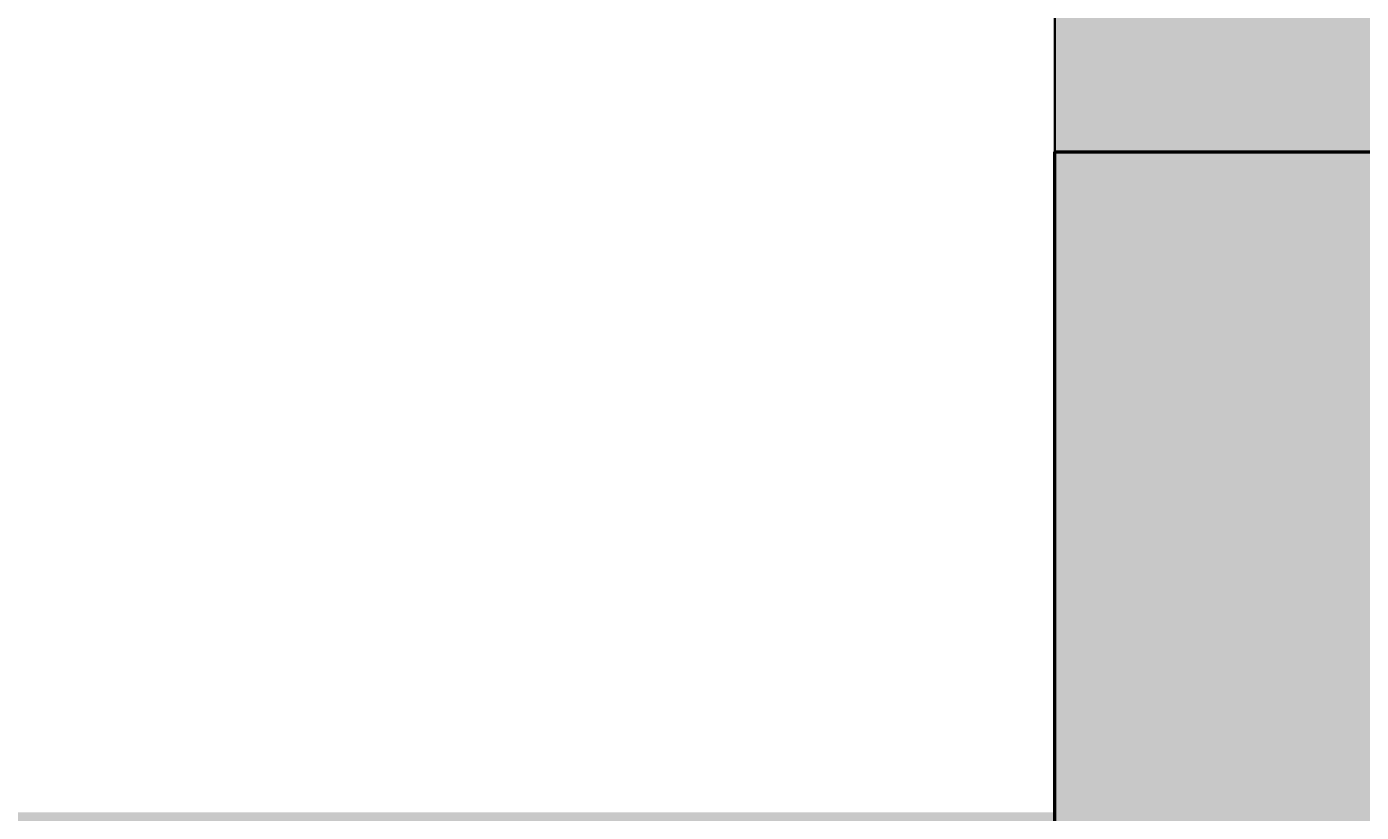
# Model space of a CAD drawing. Units: inches. Extents: x 1998 to 2588, y 1139 to 1977.
# Tile 60 of 134: x 2063 to 2095, y 1760 to 1779. Entities that reach past the tile are written whole.
import ezdxf

# ---------------------------------------------------------------- set-up
doc = ezdxf.new("R2010")
doc.units = ezdxf.units.IN
for name, color, linetype, lineweight in [('A-ANNO-DIMS', 2, 'Continuous', 18), ('A-COLS-PATT', 250, 'Continuous', 13), ('A-WALL-PATT', 252, 'Continuous', 13), ('COLUMN', 10, 'Continuous', 50), ('WALL', 200, 'Continuous', 35)]:
    doc.layers.add(name, color=color, linetype=linetype, lineweight=lineweight)
doc.styles.get("Standard").update_dxf_attribs({"font": 'arial.ttf'})
doc.dimstyles.get("Standard").update_dxf_attribs({"dimtxt": 0.18, "dimasz": 0.18, "dimexe": 0.18, "dimexo": 0.0625, "dimgap": 0.09, "dimtad": 0, "dimtih": 1, "dimtoh": 1, "dimdec": 4, "dimzin": 0, "dimdsep": 46, "dimtxsty": 'Standard', "dimcen": 0.09, "dimadec": 0, "dimazin": 0, "dimtfac": 1, "dimtdec": 4, "dimtofl": 0, "dimtmove": 0, "dimatfit": 3, "dimfxl": 1, "dimtolj": 1, "dimtzin": 0, "dimarcsym": 0})

# ---------------------------------------------------------------- blocks, each defined once
blk = doc.blocks.new('*D28')
at = {"layer": 'A-ANNO-DIMS', "color": 0, "lineweight": -2, "transparency": 16777216}
for p, q in [((2059.473, 1759.795), (2059.473, 1977.362)), ((2087.973, 1759.795), (2087.973, 1977.362)), ((2059.653, 1977.182), (2073.397, 1977.182)), ((2087.793, 1977.182), (2074.049, 1977.182))]:
    blk.add_line(p, q, dxfattribs=at)
at = {"layer": 'A-ANNO-DIMS', "color": 0, "transparency": 16777216}
for points in [[(2059.653, 1977.212), (2059.653, 1977.152), (2059.473, 1977.182)], [(2087.793, 1977.212), (2087.793, 1977.152), (2087.973, 1977.182)]]:
    blk.add_solid(points, dxfattribs=at)
at = {"layer": 'Defpoints', "color": 0, "transparency": 16777216}
for p in [(2087.973, 1977.182), (2059.473, 1759.732), (2087.973, 1759.732)]:
    blk.add_point(p, dxfattribs=at)
at = {"layer": 'A-ANNO-DIMS', "color": 0, "transparency": 16777216, "insert": (2073.723, 1977.182), "char_height": 0.18, "attachment_point": 5}
blk.add_mtext('\\A1;28.5', dxfattribs=at)
blk = doc.blocks.new('*D29')
at = {"layer": 'A-ANNO-DIMS', "color": 0, "lineweight": -2, "transparency": 16777216}
for p, q in [((2087.91, 1888.732), (1997.843, 1888.732)), ((1998.023, 1888.552), (1998.023, 1824.414)), ((1998.023, 1759.912), (1998.023, 1824.05)), ((2059.41, 1759.732), (1997.843, 1759.732))]:
    blk.add_line(p, q, dxfattribs=at)
at = {"layer": 'A-ANNO-DIMS', "color": 0, "transparency": 16777216}
for points in [[(1997.993, 1888.552), (1998.053, 1888.552), (1998.023, 1888.732)], [(1997.993, 1759.912), (1998.053, 1759.912), (1998.023, 1759.732)]]:
    blk.add_solid(points, dxfattribs=at)
at = {"layer": 'Defpoints', "color": 0, "transparency": 16777216}
for p in [(1998.023, 1888.732), (2087.973, 1888.732), (2059.473, 1759.732)]:
    blk.add_point(p, dxfattribs=at)
at = {"layer": 'A-ANNO-DIMS', "color": 0, "transparency": 16777216, "insert": (1998.023, 1824.232), "char_height": 0.18, "attachment_point": 5}
blk.add_mtext('\\A1;129', dxfattribs=at)

msp = doc.modelspace()

# ---------------------------------------------------------------- hatches: boundary and pattern name
at = {"layer": 'A-COLS-PATT'}
h = msp.add_hatch(color=256, dxfattribs=at)
h.dxf.hatch_style = 1
h.paths.add_polyline_path([(2099.4125, 1888.7324), (2087.9729, 1888.7324), (2087.9729, 1868.3278), (2099.4125, 1868.3278)])
h.paths.add_polyline_path([(2234.4125, 1888.7324), (2222.9729, 1888.7324), (2222.9729, 1868.3278), (2234.4125, 1868.3278)])
h.paths.add_polyline_path([(2341.4729, 1886.637), (2330.0332, 1886.637), (2330.0332, 1866.2324), (2341.4729, 1866.2324)])
h.paths.add_polyline_path([(2507.8006, 1882.7324), (2487.396, 1882.7324), (2487.396, 1871.2927), (2507.8006, 1871.2927)])
h.paths.add_polyline_path([(2510.9729, 1766.672), (2490.5682, 1766.672), (2490.5682, 1755.2324), (2510.9729, 1755.2324)])
h.paths.add_polyline_path([(2345.9729, 1759.7324), (2334.5332, 1759.7324), (2334.5332, 1739.3278), (2345.9729, 1739.3278)])
h.paths.add_polyline_path([(2234.4125, 1774.3318), (2222.9729, 1774.3318), (2222.9729, 1753.9272), (2234.4125, 1753.9272)])
h.paths.add_polyline_path([(2099.4125, 1775.637), (2087.9729, 1775.637), (2087.9729, 1755.2324), (2099.4125, 1755.2324)])
h.paths.add_polyline_path([(2098.0956, 1593.7241), (2077.691, 1593.7241), (2077.691, 1582.2845), (2098.0956, 1582.2845)])
h.paths.add_polyline_path([(2227.4729, 1604.637), (2216.0332, 1604.637), (2216.0332, 1584.2324), (2227.4729, 1584.2324)])
h.paths.add_polyline_path([(2345.9729, 1647.5211), (2334.5332, 1647.5211), (2334.5332, 1627.1165), (2345.9729, 1627.1165)])
h.paths.add_polyline_path([(2522.3775, 1641.2324), (2501.9729, 1641.2324), (2501.9729, 1629.7927), (2522.3775, 1629.7927)])
h.paths.add_polyline_path([(2522.3775, 1480.7324), (2501.9729, 1480.7324), (2501.9729, 1469.2927), (2522.3775, 1469.2927)])
h.paths.add_polyline_path([(2345.9729, 1488.5616), (2334.5332, 1488.5616), (2334.5332, 1468.1569), (2345.9729, 1468.1569)])
h.paths.add_polyline_path([(2234.4125, 1486.137), (2227.4729, 1486.137), (2227.4729, 1465.7324), (2234.4125, 1465.7324)])
h.paths.add_polyline_path([(2227.4729, 1486.137), (2222.9729, 1486.137), (2222.9729, 1465.7324), (2227.4729, 1465.7324)])
h.paths.add_polyline_path([(2108.3775, 1470.2324), (2087.9729, 1470.2324), (2087.9729, 1458.7927), (2108.3775, 1458.7927)])
h.paths.add_polyline_path([(2096.9729, 1365.5012), (2087.9729, 1365.5012), (2087.9729, 1345.0966), (2096.9729, 1345.0966)])
h.paths.add_polyline_path([(2087.9729, 1365.5012), (2085.5332, 1365.5012), (2085.5332, 1345.0966), (2087.9729, 1345.0966)])
h.paths.add_polyline_path([(2234.4125, 1285.137), (2222.9729, 1285.137), (2222.9729, 1264.7324), (2234.4125, 1264.7324)])
h.paths.add_polyline_path([(2345.9729, 1285.137), (2334.5332, 1285.137), (2334.5332, 1264.7324), (2345.9729, 1264.7324)])
h.paths.add_polyline_path([(2503.1458, 1240.172), (2482.7412, 1240.172), (2482.7412, 1228.7324), (2503.1458, 1228.7324)])
h.paths.add_polyline_path([(2510.9729, 1369.172), (2490.5682, 1369.172), (2490.5682, 1357.7324), (2510.9729, 1357.7324)])
at = {"layer": 'A-WALL-PATT'}
h = msp.add_hatch(color=256, dxfattribs=at)
h.dxf.hatch_style = 1
h.paths.add_polyline_path([(2222.9729, 1888.7324), (2099.4125, 1888.7324), (2099.4125, 1879.7324), (2222.9729, 1879.7324)])
h.paths.add_polyline_path([(2096.9729, 1868.3278), (2087.9729, 1868.3278), (2087.9729, 1775.637), (2096.9729, 1775.637)])
h.paths.add_polyline_path([(2227.4729, 1868.3278), (2222.9729, 1868.3278), (2222.9729, 1774.3318), (2227.4729, 1774.3318)])
h.paths.add_polyline_path([(2188.3019, 1759.7324), (2138.6074, 1759.7324), (2099.4125, 1759.7324), (2099.4125, 1755.2324), (2176.9729, 1755.2324), (2188.3019, 1755.2324)])
h.paths.add_polyline_path([(2087.9729, 1759.7324), (2059.4729, 1759.7324), (2059.4729, 1702.7324), (2087.9729, 1702.7324), (2087.9729, 1707.2324), (2063.9729, 1707.2324), (2063.9729, 1755.2324), (2087.9729, 1755.2324)])
h.paths.add_polyline_path([(2096.9729, 1755.2324), (2087.9729, 1755.2324), (2087.9729, 1707.2324), (2096.9729, 1707.2324)])
h.paths.add_polyline_path([(2187.0461, 1707.2324), (2105.9729, 1707.2324), (2096.9729, 1707.2324), (2087.9729, 1707.2324), (2087.9729, 1702.7324), (2105.9729, 1702.7324), (2114.9729, 1702.7324), (2187.0461, 1702.7324)])
h.paths.add_polyline_path([(2181.4729, 1719.2028), (2176.9729, 1719.2028), (2176.9729, 1707.2324), (2181.4729, 1707.2324)])
h.paths.add_polyline_path([(2216.0332, 1588.7324), (2114.9729, 1588.7324), (2105.9729, 1588.7324), (2105.9729, 1584.2324), (2216.0332, 1584.2324)])
h.paths.add_polyline_path([(2077.691, 1588.7324), (2061.4729, 1588.7324), (2061.4729, 1584.2324), (2077.691, 1584.2324)])
h.paths.add_polyline_path([(2105.9729, 1588.7324), (2098.0956, 1588.7324), (2098.0956, 1584.2324), (2105.9729, 1584.2324)])
h.paths.add_polyline_path([(2114.9729, 1596.2642), (2110.1012, 1596.2642), (2105.9729, 1596.2642), (2105.9729, 1588.7324), (2114.9729, 1588.7324)])
h.paths.add_polyline_path([(2114.9729, 1584.2324), (2105.9729, 1584.2324), (2105.9729, 1580.249), (2110.1012, 1580.249), (2114.9729, 1580.249)])
h.paths.add_polyline_path([(2114.9729, 1547.7716), (2110.1012, 1547.7716, -0.0318759), (2105.9729, 1548.035), (2105.9729, 1470.2324), (2108.3775, 1470.2324), (2108.3775, 1465.7324), (2186.2943, 1465.7324), (2186.2943, 1470.2324), (2114.9729, 1470.2324)])
h.paths.add_polyline_path([(2227.4729, 1584.2324), (2222.9729, 1584.2324), (2222.9729, 1486.137), (2227.4729, 1486.137)])
h.paths.add_polyline_path([(2295.4138, 1593.2324), (2227.4729, 1593.2324), (2227.4729, 1588.7324), (2295.4138, 1588.7324), (2295.4138, 1591.8729)])
h.paths.add_polyline_path([(2345.9729, 1627.1165), (2341.4729, 1627.1165), (2341.4729, 1593.2324), (2337.2869, 1593.2324), (2337.2869, 1591.8729), (2337.2869, 1588.7324), (2345.9729, 1588.7324)])
h.paths.add_polyline_path([(2291.9729, 1588.7324), (2287.4729, 1588.7324), (2287.4729, 1522.7324), (2291.9729, 1522.7324)])
h.paths.add_polyline_path([(2291.9729, 1522.7324), (2287.4729, 1522.7324), (2227.4729, 1522.7324), (2227.4729, 1518.2324), (2291.9729, 1518.2324)])
h.paths.add_polyline_path([(2295.7347, 1519.5919), (2295.7347, 1522.7324), (2291.9729, 1522.7324), (2291.9729, 1518.2324), (2295.7347, 1518.2324)])
h.paths.add_polyline_path([(2345.9729, 1522.7324), (2337.6078, 1522.7324), (2337.6078, 1519.5919), (2337.6078, 1518.2324), (2341.4729, 1518.2324), (2341.4729, 1488.5616), (2345.9729, 1488.5616)])
h.paths.add_polyline_path([(2345.9729, 1468.1569), (2341.4729, 1468.1569), (2341.4729, 1374.2324), (2227.4729, 1374.2324), (2227.4729, 1369.7324), (2345.9729, 1369.7324)])
h.paths.add_polyline_path([(2345.9729, 1369.7324), (2341.4729, 1369.7324), (2341.4729, 1362.2324), (2345.9729, 1362.2324)])
h.paths.add_polyline_path([(2345.9729, 1317.7324), (2345.9729, 1322.2324), (2341.4729, 1322.2324), (2341.4729, 1285.137), (2345.9729, 1285.137)], flags=17)
h.paths.add_polyline_path([(2356.2096, 1322.2324), (2345.9729, 1322.2324), (2345.9729, 1317.7324), (2356.2096, 1317.7324), (2356.2096, 1319.3088)], flags=17)
h.paths.add_polyline_path([(2393.9729, 1322.2324), (2375.6999, 1322.2324), (2375.6999, 1319.3088, -0.0202458), (2375.636, 1317.7324), (2393.9729, 1317.7324)], flags=17)
h.paths.add_polyline_path([(2398.4729, 1322.2324), (2393.9729, 1322.2324), (2393.9729, 1317.7324), (2393.9729, 1237.7324), (2345.9729, 1237.7324), (2345.9729, 1264.7324), (2341.4729, 1264.7324), (2341.4729, 1228.7324), (2393.9729, 1228.7324), (2482.7412, 1228.7324), (2482.7412, 1237.7324), (2398.4729, 1237.7324), (2398.4729, 1297.1029)])
h.paths.add_polyline_path([(2398.4729, 1362.2324), (2393.9729, 1362.2324), (2393.9729, 1357.7324), (2398.4729, 1357.7324)])
h.paths.add_polyline_path([(2345.9729, 1329.7549), (2341.4729, 1329.7549), (2341.4729, 1322.2324), (2345.9729, 1322.2324)])

# ---------------------------------------------------------------- linework, layer by layer
at = {"layer": 'COLUMN'}
msp.add_lwpolyline([(2087.9729, 1775.637), (2099.4125, 1775.637), (2099.4125, 1755.2324), (2087.9729, 1755.2324)], close=True, dxfattribs=at)
at = {"layer": 'WALL'}
msp.add_line((2087.9729, 1888.7324), (2087.9729, 1755.2324), dxfattribs=at)

# ---------------------------------------------------------------- dimensions: what is measured, and where the dimension line sits
at = {"layer": 'A-ANNO-DIMS'}
dim = msp.add_linear_dim(base=(2087.9729, 1977.1824), p1=(2059.4729, 1759.7324), p2=(2087.9729, 1759.7324), dimstyle='Standard', override={"dimdec": 1, "dimlfac": 1, "dimrnd": 0, "dimzin": 0, "dimdsep": 46, "dimlunit": 2}, dxfattribs=at)
dim.commit()
dim.dimension.update_dxf_attribs({"geometry": '*D28', "text_midpoint": (2073.7229, 1977.1824)})
dim = msp.add_linear_dim(base=(1998.0229, 1888.7324), p1=(2059.4729, 1759.7324), p2=(2087.9729, 1888.7324), angle=90, dimstyle='Standard', override={"dimdec": 0, "dimlfac": 1, "dimrnd": 0, "dimzin": 0, "dimdsep": 46, "dimlunit": 2}, dxfattribs=at)
dim.commit()
dim.dimension.update_dxf_attribs({"geometry": '*D29', "text_midpoint": (1998.0229, 1824.2324)})

doc.saveas('drawing.dxf')
